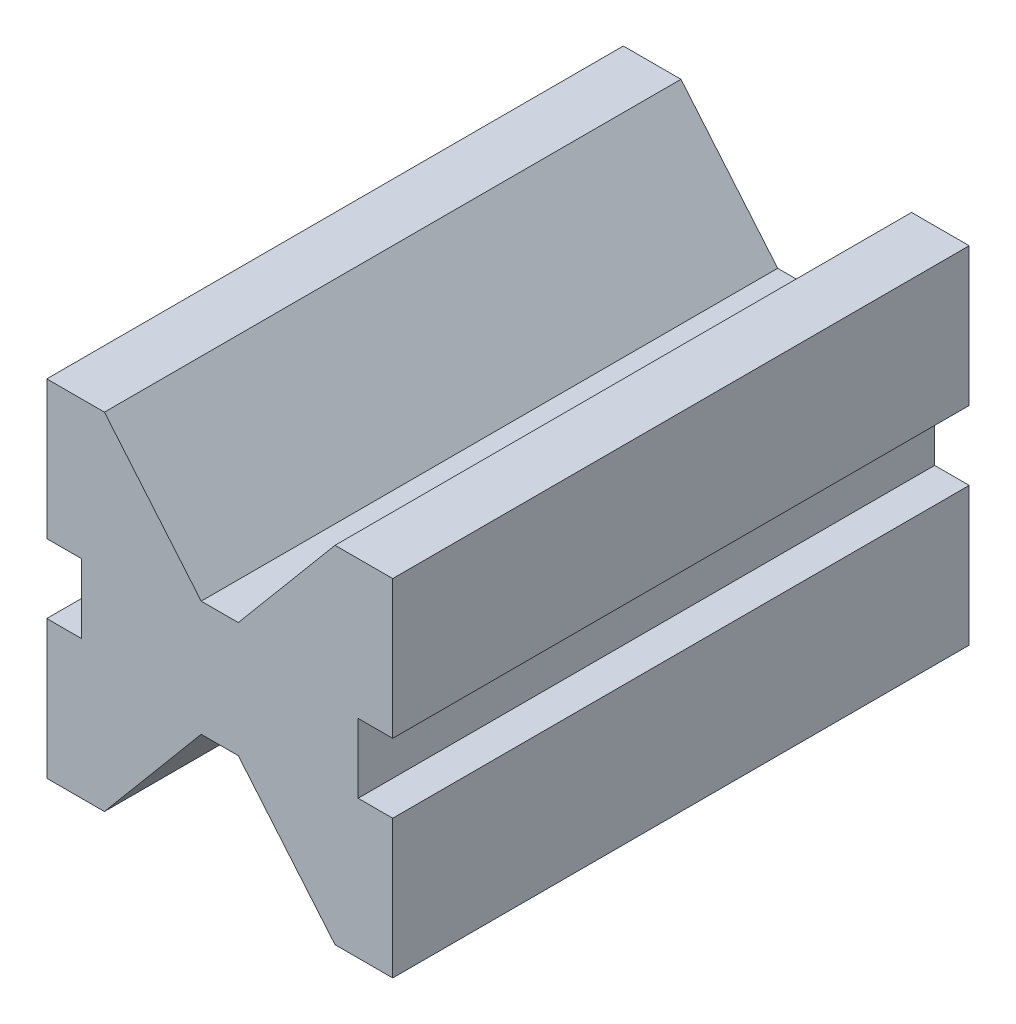
SolidWorks part; units mm, degrees
material "Plain Carbon Steel"
ref_plane "Front Plane" through (0, 0, 0) normal (0, 0, 1) x (1, 0, 0)
ref_plane "Top Plane" through (0, 0, 0) normal (0, 1, 0) x (1, 0, 0)
ref_plane "Right Plane" through (0, 0, 0) normal (1, 0, 0) x (0, 0, -1)
sketch "V-Block Profile Sketch" plane through (0, 0, 0) normal (0, 0, 1) x (1, 0, 0)
  line L0 (-30, -30) -> (-30, -6)
  line L1 (30, 6) -> (30, 30)
  line L2 (30, 30) -> (20, 30)
  line L3 (-30, 30) -> (-30, 6)
  line L4 (-30, -30) -> (-20, -30)
  line L5 (30, -30) -> (30, -6)
  line L6 (-30, -6) -> (-24, -6)
  line L7 (-30, 30) -> (-30, 6)
  line L8 (-30, 6) -> (-24, 6)
  line L9 (-24, 6) -> (-24, -6)
  line L10 (-30, -6) -> (-30, -30)
  line L11 (30, 6) -> (24, 6)
  line L12 (24, 6) -> (24, -6)
  line L13 (24, -6) -> (30, -6)
  line L15 (0, -10) -> (3.218, -10)
  line L16 (0, -10) -> (-3.218, -10)
  line L18 (20, -30) -> (30, -30)
  line L20 (20, -30) -> (3.218, -10)
  line L22 (-20, -30) -> (-3.1213, -9.8847)
  line L23 (20, 30) -> (3.218, 10)
  line L24 (0, 10) -> (-3.218, 10)
  line L25 (0, 10) -> (3.218, 10)
  line L26 (-20, 30) -> (-3.1213, 9.8847)
  line L27 (-20, 30) -> (-30, 30)
  dimension "D1" = 60
  dimension "D2" = 60
  dimension "D3" = 30
  dimension "D4" = 16.8787
  dimension "D5" = 50
  dimension "D6" = 24
  dimension "D7" = 10
  dimension "D8" = 24
  dimension "D9" = 12
  dimension "D10" = 6
  dimension "D11" = 48
  dimension "D12" = 16.782
  dimension "D13" = 16.8787
  dimension "D14" = 16.782
  dimension "D15" = 3.9627
  dimension "D16" = 140
  dimension "D17" = 40
  dimension "D18" = 6.436
  dimension "D19" = 6.3393
  dimension "D20" = 108.88
  dimension "D21" = 140
  dimension "D22" = 3.9627
  dimension "D23" = 3.9627
  dimension "D24" = 144.324
  dimension "D25" = 3.218
  dimension "D26" = 90
extrude "V-Block Body Extrude 100" add sketch "V-Block Profile Sketch" against normal blind 100
ref_plane "Plane1" through (0, 0, -60) normal (0, 0, 1) x (1, 0, 0)
